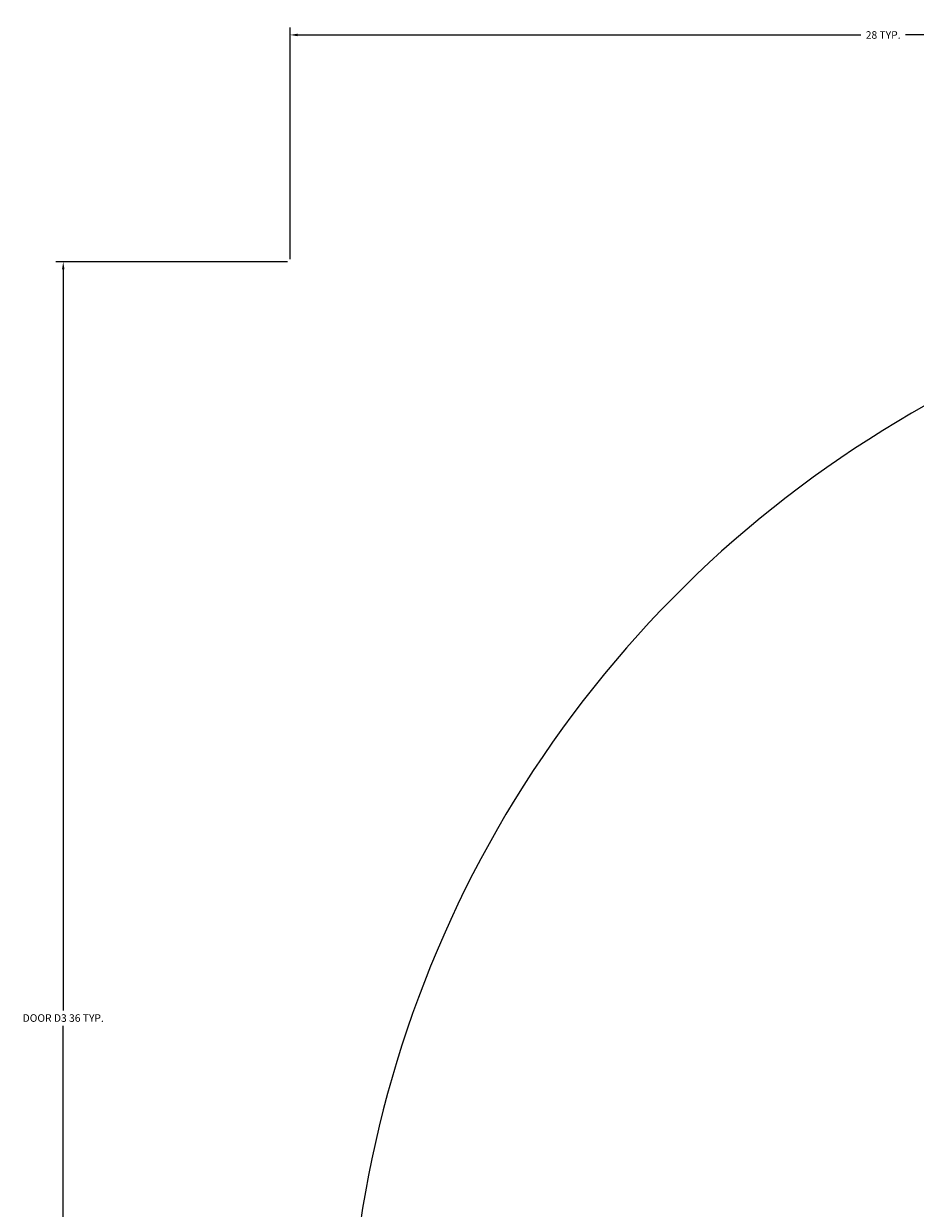
# Model space of a CAD drawing. Units: inches. Extents: x 1901 to 2863, y 888 to 2433.
# Tile 76 of 91: x 2564 to 2586, y 2094 to 2123. Entities that reach past the tile are written whole.
import ezdxf

# ---------------------------------------------------------------- set-up
doc = ezdxf.new("R2010")
doc.units = ezdxf.units.IN
doc.layers.add('A-ANNO-DIMS', color=2, linetype='Continuous', lineweight=18)
doc.layers.add('A-DOOR', color=4, linetype='Continuous', lineweight=25)
doc.styles.get("Standard").update_dxf_attribs({"font": 'arial.ttf'})
doc.dimstyles.get("Standard").update_dxf_attribs({"dimtxt": 0.18, "dimasz": 0.18, "dimexe": 0.18, "dimexo": 0.0625, "dimgap": 0.09, "dimtad": 0, "dimtih": 1, "dimtoh": 1, "dimdec": 4, "dimzin": 0, "dimdsep": 46, "dimtxsty": 'Standard', "dimcen": 0.09, "dimadec": 0, "dimazin": 0, "dimtfac": 1, "dimtdec": 4, "dimtofl": 0, "dimtmove": 0, "dimatfit": 3, "dimfxl": 1, "dimtolj": 1, "dimtzin": 0, "dimarcsym": 0})

# ---------------------------------------------------------------- blocks, each defined once
blk = doc.blocks.new('DOOR-27')
blk.add_arc((26.814, 9.122), 26.862, 90, 199.8893)
blk = doc.blocks.new('*D35')
at = {"layer": 'A-ANNO-DIMS', "color": 0, "lineweight": -2, "transparency": 16777216}
for p, q in [((2570.714, 2116.884), (2565.196, 2116.884)), ((2565.376, 2116.704), (2565.376, 2099.067)), ((2565.376, 2081.064), (2565.376, 2098.701)), ((2570.714, 2080.884), (2565.196, 2080.884))]:
    blk.add_line(p, q, dxfattribs=at)
at = {"layer": 'A-ANNO-DIMS', "color": 0, "transparency": 16777216}
for points in [[(2565.346, 2116.704), (2565.406, 2116.704), (2565.376, 2116.884)], [(2565.346, 2081.064), (2565.406, 2081.064), (2565.376, 2080.884)]]:
    blk.add_solid(points, dxfattribs=at)
at = {"layer": 'Defpoints', "color": 0, "transparency": 16777216}
for p in [(2565.376, 2116.884), (2570.776, 2116.884), (2570.776, 2080.884)]:
    blk.add_point(p, dxfattribs=at)
at = {"layer": 'A-ANNO-DIMS', "color": 0, "transparency": 16777216, "insert": (2565.376, 2098.884), "char_height": 0.18, "attachment_point": 5}
blk.add_mtext('\\A1;DOOR D3 36 TYP.', dxfattribs=at)
blk = doc.blocks.new('*D36')
at = {"layer": 'A-ANNO-DIMS', "color": 0, "lineweight": -2, "transparency": 16777216}
for p, q in [((2570.776, 2116.946), (2570.776, 2122.464)), ((2599.014, 2116.946), (2599.014, 2122.464)), ((2570.956, 2122.284), (2584.366, 2122.284)), ((2598.834, 2122.284), (2585.425, 2122.284))]:
    blk.add_line(p, q, dxfattribs=at)
at = {"layer": 'A-ANNO-DIMS', "color": 0, "transparency": 16777216}
for points in [[(2570.956, 2122.314), (2570.956, 2122.254), (2570.776, 2122.284)], [(2598.834, 2122.314), (2598.834, 2122.254), (2599.014, 2122.284)]]:
    blk.add_solid(points, dxfattribs=at)
at = {"layer": 'Defpoints', "color": 0, "transparency": 16777216}
for p in [(2599.014, 2122.284), (2570.776, 2116.884), (2599.014, 2116.884)]:
    blk.add_point(p, dxfattribs=at)
at = {"layer": 'A-ANNO-DIMS', "color": 0, "transparency": 16777216, "insert": (2584.895, 2122.284), "char_height": 0.18, "attachment_point": 5}
blk.add_mtext('\\A1;28 TYP.', dxfattribs=at)

msp = doc.modelspace()

# ---------------------------------------------------------------- block references
at = {"layer": 'A-DOOR'}
msp.add_blockref('DOOR-27', (2572.2, 2080.9), dxfattribs=at)

# ---------------------------------------------------------------- dimensions: what is measured, and where the dimension line sits
at = {"layer": 'A-ANNO-DIMS'}
dim = msp.add_linear_dim(base=(2599.014, 2122.284), p1=(2570.776, 2116.884), p2=(2599.014, 2116.884), text='<> TYP.', dimstyle='Standard', override={"dimdec": 0, "dimlfac": 1, "dimrnd": 0, "dimzin": 0, "dimdsep": 46, "dimlunit": 2}, dxfattribs=at)
dim.commit()
dim.dimension.update_dxf_attribs({"geometry": '*D36', "text_midpoint": (2584.895, 2122.284)})
dim = msp.add_linear_dim(base=(2565.376, 2116.884), p1=(2570.776, 2080.884), p2=(2570.776, 2116.884), angle=90, text='DOOR D3 <> TYP.', dimstyle='Standard', override={"dimdec": 0, "dimlfac": 1, "dimrnd": 0, "dimzin": 0, "dimdsep": 46, "dimlunit": 2}, dxfattribs=at)
dim.commit()
dim.dimension.update_dxf_attribs({"geometry": '*D35', "text_midpoint": (2565.376, 2098.884)})

doc.saveas('drawing.dxf')
